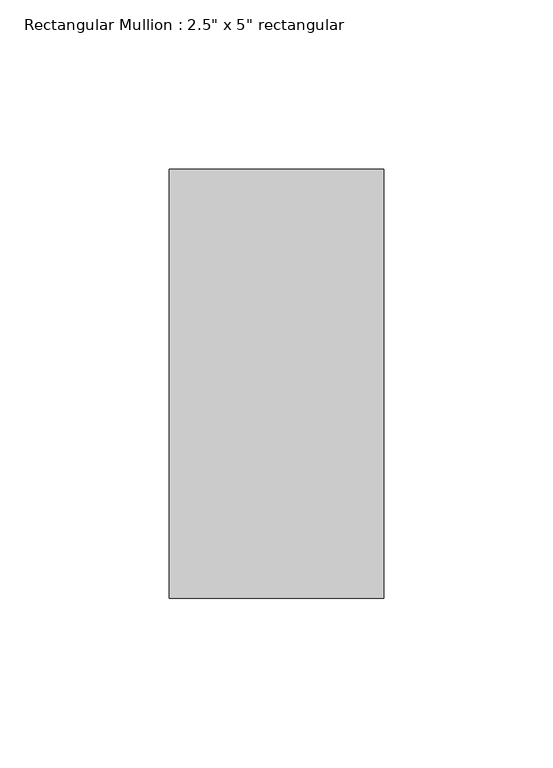
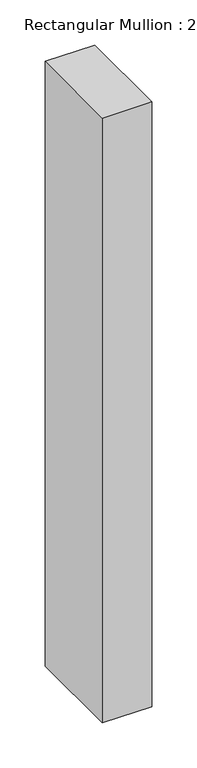
"""IFC4 building model written with IfcOpenShell, lengths in millimetres: member geometry."""

from ifc_helpers import new_model, si_unit, frame, origin, place, context, project, spatial, polyline, outline, extrude, source, transform, mapped, element, save


def member_8d24a278(model_context):
    return source(origin(), model_context, "Body", "SweptSolid", [
        extrude(outline(polyline([(0.0, 63.5), (0.0, -63.5), (-63.5, -63.5), (-63.5, 63.5), (0.0, 63.5)])), frame((0.0, 0.0, -818.8529818), z_axis=(0.0, 0.0, 1.0), x_axis=(1.0, 0.0, 0.0)), (0.0, 0.0, 1.0), 818.8529818),
    ])


if __name__ == "__main__":
    model = new_model("IFC4")
    model_context = context("Model", 3, world=origin())
    ifc_project = project(units=[si_unit("LENGTHUNIT", "METRE", prefix="MILLI")], contexts=[model_context])
    site = spatial("IfcSite", under=ifc_project)
    building = spatial("IfcBuilding", under=site)
    placement = place(None, origin())
    member_shape = member_8d24a278(model_context)
    element("IfcMember", 1, ObjectType="Rectangular Mullion : 2.5\" x 5\" rectangular", at=placement, inside=building, context=model_context, shape_type="MappedRepresentation", body=[
        mapped(member_shape, transform((0.0, 0.0, 0.0), x_axis=(1.0, 0.0, 0.0), y_axis=(0.0, 1.0, 0.0), z_axis=(0.0, 0.0, 1.0))),
    ])
    save(model, "model.ifc")

# Revit data of these elements
# Type "Rectangular Mullion : 2.5\" x 5\" rectangular"
#   built-in parameter 1007304 = 0.416667 (stored number, unit not read)
#   built-in parameter 1007301 = 0.104167 (stored number, unit not read)
#   built-in parameter 1007300 = 0.104167 (stored number, unit not read)
# Element 1 (IfcMember, "Rectangular Mullion : 2.5\" x 5\" rectangular")
#   Materials on its faces: "Aluminum"
# Materials
#   "Aluminum": class "Metal", colour RGB 247 247 247, transparency 0, Description = "Aluminum 6061", Cost = 0
